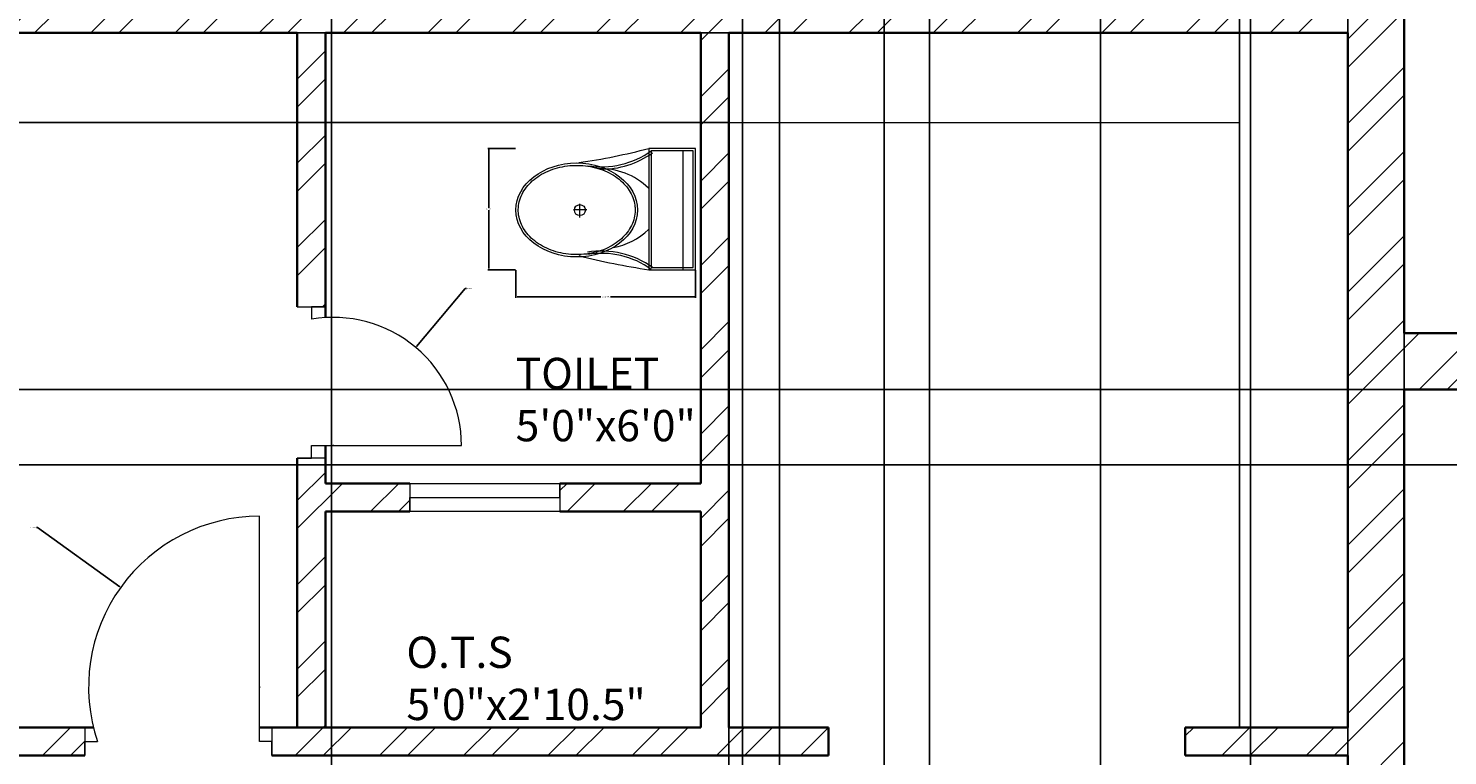
# Model space of a CAD drawing. Units: inches. Extents: x 1748 to 2382, y 1346 to 2284.
# Tile 11 of 26: x 1920 to 2147, y 1855 to 1971. Entities that reach past the tile are written whole.
import ezdxf

# ---------------------------------------------------------------- set-up
doc = ezdxf.new("R2010")
doc.units = ezdxf.units.IN
for name, color, linetype, lineweight in [('A-ANNO-DIMS', 2, 'Continuous', 18), ('A-AREA-IDEN', 7, 'Continuous', 18), ('A-DOOR', 21, 'Continuous', 18), ('A-FLOR-CASE', 32, 'Continuous', 18), ('A-FLOR-FIXT', 7, 'Continuous', 18), ('A-GLAZ', 191, 'Continuous', 18), ('A-WALL', 7, 'Continuous', 35), ('A-WALL-PATT', 9, 'Continuous', 13)]:
    doc.layers.add(name, color=color, linetype=linetype, lineweight=lineweight)
doc.styles.get("Standard").update_dxf_attribs({"font": 'arial.ttf'})
doc.dimstyles.get("Standard").update_dxf_attribs({"dimtxt": 0.18, "dimasz": 0.18, "dimexe": 0.18, "dimexo": 0.0625, "dimgap": 0.09, "dimtad": 0, "dimtih": 1, "dimtoh": 1, "dimdec": 4, "dimzin": 0, "dimdsep": 46, "dimtxsty": 'Standard', "dimcen": 0.09, "dimadec": 0, "dimazin": 0, "dimtfac": 1, "dimtdec": 4, "dimtofl": 0, "dimtmove": 0, "dimatfit": 3, "dimfxl": 1, "dimtolj": 1, "dimtzin": 0, "dimarcsym": 0})

# ---------------------------------------------------------------- blocks, each defined once
blk = doc.blocks.new('A$C31115884')
for p, q in [((283.1, 497.7), (223.4, 497.7)), ((257.5, 466.4), (257.5, 523.2)), ((0, 200), (0, 0)), ((520, 200), (0, 200)), ((10, 190), (10, 10)), ((510, 190), (10, 190)), ((510, 10), (510, 190)), ((520, 0), (520, 200)), ((510, 54.5), (0, 54.5)), ((10, 10), (510, 10)), ((0, 0), (520, 0))]:
    blk.add_line(p, q)
blk.add_circle((255.6, 496.4), 23.6)
for centre, radius, start, end in [((2777.7, -204.6), 2807, 165.4549, 171.71327), ((3237, 905), 2807, 188.28673, 194.5451), ((-294.5, 403.3), 364.7, 324.20913, 9.34987), ((-294.5, 403.3), 374.7, 324.20913, 9.34987), ((805.8, 403.3), 364.7, 170.65013, 215.79087), ((139.5, 406.2), 293.5, 315.84364, 2.65635), ((805.8, 403.3), 374.7, 179.20365, 215.79087), ((383.6, 406.2), 293.5, 190.27735, 224.15636)]:
    blk.add_arc(centre, radius, start, end)
blk.add_ellipse((256.2, 509.9), major_axis=(0, -260.7), ratio=0.772727)
blk.add_open_spline([(256.2, 259.2), (263.1, 259.2), (270, 259.7), (287.8, 262.3), (298.7, 265.1), (319.9, 273.1), (330.2, 278.4), (350.1, 291.1), (359.7, 298.7), (377.7, 315.9), (386.2, 325.5), (401.7, 346.6), (408.8, 358.1), (421.3, 382.5), (426.8, 395.5), (435.9, 422.4), (439.5, 436.4), (444.8, 465.1), (446.5, 479.7), (447.9, 509.2), (447.6, 524), (445, 553.3), (442.7, 567.8), (436.3, 596), (432.1, 609.7), (421.9, 636), (416, 648.6), (402.5, 672.1), (395, 683), (378.6, 703), (369.8, 712.1), (351.1, 728), (341.3, 734.8), (320.9, 746.2), (310.4, 750.7), (288.9, 757.3), (278, 759.4), (256, 761), (245, 760.6), (223.1, 757.2), (212.3, 754.3), (191.1, 746.1), (180.8, 740.7), (160.9, 727.8), (151.4, 720.1), (133.5, 702.7), (125.1, 693), (109.6, 671.7), (102.6, 660.2), (90.2, 635.7), (84.9, 622.7), (76, 595.6), (72.4, 581.6), (67.2, 552.9), (65.6, 538.2), (64.4, 508.8), (64.8, 494), (67.5, 464.7), (69.9, 450.2), (76.6, 422), (80.8, 408.3), (91.1, 382.2), (97.2, 369.7), (110.8, 346.3), (118.4, 335.4), (134.8, 315.6), (143.7, 306.7), (162.4, 290.9), (172.3, 284.2), (192.8, 273), (203.3, 268.6), (224.8, 262.2), (235.8, 260.2), (249.9, 259.3), (253, 259.2), (256.2, 259.2)], degree=3, knots=[0, 0, 0, 0, 0.110105, 0.110105, 0.285049, 0.285049, 0.459994, 0.459994, 0.634938, 0.634938, 0.809882, 0.809882, 0.984827, 0.984827, 1.159771, 1.159771, 1.334715, 1.334715, 1.50966, 1.50966, 1.684604, 1.684604, 1.859549, 1.859549, 2.034493, 2.034493, 2.209437, 2.209437, 2.384382, 2.384382, 2.559326, 2.559326, 2.73427, 2.73427, 2.909215, 2.909215, 3.084159, 3.084159, 3.259103, 3.259103, 3.434048, 3.434048, 3.608992, 3.608992, 3.783936, 3.783936, 3.958881, 3.958881, 4.133825, 4.133825, 4.30877, 4.30877, 4.483714, 4.483714, 4.658658, 4.658658, 4.833603, 4.833603, 5.008547, 5.008547, 5.183491, 5.183491, 5.358436, 5.358436, 5.53338, 5.53338, 5.708324, 5.708324, 5.883269, 5.883269, 6.058213, 6.058213, 6.233158, 6.233158, 6.283185, 6.283185, 6.283185, 6.283185])
blk = doc.blocks.new('*D14')
at = {"layer": 'A-ANNO-DIMS', "color": 0, "lineweight": -2, "transparency": 16777216}
for p, q in [((1997.92, 1932.42), (1997.92, 1928)), ((2026.64, 1932.42), (2026.64, 1928)), ((1998.1, 1928.18), (2011.5, 1928.18)), ((2026.46, 1928.18), (2013.06, 1928.18))]:
    blk.add_line(p, q, dxfattribs=at)
at = {"layer": 'A-ANNO-DIMS', "color": 0, "transparency": 16777216}
for points in [[(1998.1, 1928.21), (1998.1, 1928.15), (1997.92, 1928.18)], [(2026.46, 1928.21), (2026.46, 1928.15), (2026.64, 1928.18)]]:
    blk.add_solid(points, dxfattribs=at)
at = {"layer": 'Defpoints', "color": 0, "transparency": 16777216}
for p in [(1997.92, 1932.48), (2026.64, 1932.48), (1997.92, 1928.18)]:
    blk.add_point(p, dxfattribs=at)
at = {"layer": 'A-ANNO-DIMS', "color": 0, "transparency": 16777216, "insert": (2012.28, 1928.18), "char_height": 0.18, "attachment_point": 5}
blk.add_mtext('\\A1;WC 29 TYP.', dxfattribs=at)
blk = doc.blocks.new('*D15')
at = {"layer": 'A-ANNO-DIMS', "color": 0, "lineweight": -2, "transparency": 16777216}
for p, q in [((1997.86, 1951.87), (1993.43, 1951.87)), ((1993.61, 1951.69), (1993.61, 1942.36)), ((1993.61, 1932.66), (1993.61, 1941.99)), ((1997.86, 1932.48), (1993.43, 1932.48))]:
    blk.add_line(p, q, dxfattribs=at)
at = {"layer": 'A-ANNO-DIMS', "color": 0, "transparency": 16777216}
for points in [[(1993.58, 1951.69), (1993.64, 1951.69), (1993.61, 1951.87)], [(1993.58, 1932.66), (1993.64, 1932.66), (1993.61, 1932.48)]]:
    blk.add_solid(points, dxfattribs=at)
at = {"layer": 'Defpoints', "color": 0, "transparency": 16777216}
for p in [(1993.61, 1951.87), (1997.92, 1951.87), (1997.92, 1932.48)]:
    blk.add_point(p, dxfattribs=at)
at = {"layer": 'A-ANNO-DIMS', "color": 0, "transparency": 16777216, "insert": (1993.61, 1942.18), "char_height": 0.18, "attachment_point": 5}
blk.add_mtext('\\A1;19 TYP.', dxfattribs=at)
blk = doc.blocks.new('*D36')
at = {"layer": 'A-ANNO-DIMS', "color": 0, "lineweight": -2, "transparency": 16777216}
for p, q in [((2031.96, 1970.29), (2031.96, 1360.47)), ((2130.96, 1970.29), (2130.96, 1360.47)), ((2032.14, 1360.65), (2081.24, 1360.65)), ((2130.78, 1360.65), (2081.68, 1360.65))]:
    blk.add_line(p, q, dxfattribs=at)
at = {"layer": 'A-ANNO-DIMS', "color": 0, "transparency": 16777216}
for points in [[(2032.14, 1360.68), (2032.14, 1360.62), (2031.96, 1360.65)], [(2130.78, 1360.68), (2130.78, 1360.62), (2130.96, 1360.65)]]:
    blk.add_solid(points, dxfattribs=at)
at = {"layer": 'Defpoints', "color": 0, "transparency": 16777216}
for p in [(2031.96, 1970.35), (2130.96, 1970.35), (2130.96, 1360.65)]:
    blk.add_point(p, dxfattribs=at)
at = {"layer": 'A-ANNO-DIMS', "color": 0, "transparency": 16777216, "insert": (2081.46, 1360.65), "char_height": 0.18, "attachment_point": 5}
blk.add_mtext('\\A1;99', dxfattribs=at)
blk = doc.blocks.new('*D37')
at = {"layer": 'A-ANNO-DIMS', "color": 0, "lineweight": -2, "transparency": 16777216}
for p, q in [((2031.9, 1970.35), (1779.88, 1970.35)), ((1780.06, 1970.17), (1780.06, 1963.37)), ((1780.06, 1956.2), (1780.06, 1963.01)), ((2031.9, 1956.02), (1779.88, 1956.02))]:
    blk.add_line(p, q, dxfattribs=at)
at = {"layer": 'A-ANNO-DIMS', "color": 0, "transparency": 16777216}
for points in [[(1780.03, 1970.17), (1780.09, 1970.17), (1780.06, 1970.35)], [(1780.03, 1956.2), (1780.09, 1956.2), (1780.06, 1956.02)]]:
    blk.add_solid(points, dxfattribs=at)
at = {"layer": 'Defpoints', "color": 0, "transparency": 16777216}
for p in [(1780.06, 1970.35), (2031.96, 1970.35), (2031.96, 1956.02)]:
    blk.add_point(p, dxfattribs=at)
at = {"layer": 'A-ANNO-DIMS', "color": 0, "transparency": 16777216, "insert": (1780.06, 1963.19), "char_height": 0.18, "attachment_point": 5}
blk.add_mtext('\\A1;14.325', dxfattribs=at)
blk = doc.blocks.new('*D38')
at = {"layer": 'A-ANNO-DIMS', "color": 0, "lineweight": -2, "transparency": 16777216}
for p, q in [((2113.63, 1859.41), (2113.63, 2274.93)), ((2113.81, 2274.75), (2121.84, 2274.75)), ((2130.78, 2274.75), (2122.75, 2274.75)), ((2130.96, 1859.41), (2130.96, 2274.93))]:
    blk.add_line(p, q, dxfattribs=at)
at = {"layer": 'A-ANNO-DIMS', "color": 0, "transparency": 16777216}
for points in [[(2113.81, 2274.78), (2113.81, 2274.72), (2113.63, 2274.75)], [(2130.78, 2274.78), (2130.78, 2274.72), (2130.96, 2274.75)]]:
    blk.add_solid(points, dxfattribs=at)
at = {"layer": 'Defpoints', "color": 0, "transparency": 16777216}
for p in [(2130.96, 2274.75), (2113.63, 1859.35), (2130.96, 1859.35)]:
    blk.add_point(p, dxfattribs=at)
at = {"layer": 'A-ANNO-DIMS', "color": 0, "transparency": 16777216, "insert": (2122.29, 2274.75), "char_height": 0.18, "attachment_point": 5}
blk.add_mtext('\\A1;17.334', dxfattribs=at)
blk = doc.blocks.new('*D39')
at = {"layer": 'A-ANNO-DIMS', "color": 0, "lineweight": -2, "transparency": 16777216}
for p, q in [((2139.96, 1734.91), (2139.96, 2274.93)), ((2140.14, 2274.75), (2168.14, 2274.75)), ((2196.89, 2274.75), (2168.89, 2274.75)), ((2197.07, 1734.91), (2197.07, 2274.93))]:
    blk.add_line(p, q, dxfattribs=at)
at = {"layer": 'A-ANNO-DIMS', "color": 0, "transparency": 16777216}
for points in [[(2140.14, 2274.78), (2140.14, 2274.72), (2139.96, 2274.75)], [(2196.89, 2274.78), (2196.89, 2274.72), (2197.07, 2274.75)]]:
    blk.add_solid(points, dxfattribs=at)
at = {"layer": 'Defpoints', "color": 0, "transparency": 16777216}
for p in [(2197.07, 2274.75), (2139.96, 1734.85), (2197.07, 1734.85)]:
    blk.add_point(p, dxfattribs=at)
at = {"layer": 'A-ANNO-DIMS', "color": 0, "transparency": 16777216, "insert": (2168.52, 2274.75), "char_height": 0.18, "attachment_point": 5}
blk.add_mtext('\\A1;57.11', dxfattribs=at)
blk = doc.blocks.new('*D51')
at = {"layer": 'A-ANNO-DIMS', "color": 0, "lineweight": -2, "transparency": 16777216}
for p, q in [((1968.44, 2223.79), (1968.44, 1360.47)), ((2040.07, 2223.79), (2040.07, 1360.47)), ((1968.62, 1360.65), (2003.86, 1360.65)), ((2039.89, 1360.65), (2004.65, 1360.65))]:
    blk.add_line(p, q, dxfattribs=at)
at = {"layer": 'A-ANNO-DIMS', "color": 0, "transparency": 16777216}
for points in [[(1968.62, 1360.68), (1968.62, 1360.62), (1968.44, 1360.65)], [(2039.89, 1360.68), (2039.89, 1360.62), (2040.07, 1360.65)]]:
    blk.add_solid(points, dxfattribs=at)
at = {"layer": 'Defpoints', "color": 0, "transparency": 16777216}
for p in [(1968.44, 2223.85), (2040.07, 2223.85), (2040.07, 1360.65)]:
    blk.add_point(p, dxfattribs=at)
at = {"layer": 'A-ANNO-DIMS', "color": 0, "transparency": 16777216, "insert": (2004.26, 1360.65), "char_height": 0.18, "attachment_point": 5}
blk.add_mtext('\\A1;71.62', dxfattribs=at)
blk = doc.blocks.new('*D52')
at = {"layer": 'A-ANNO-DIMS', "color": 0, "lineweight": -2, "transparency": 16777216}
for p, q in [((2064.07, 2223.79), (2064.07, 1360.47)), ((2091.4, 2223.79), (2091.4, 1360.47)), ((2064.25, 1360.65), (2077.34, 1360.65)), ((2091.22, 1360.65), (2078.13, 1360.65))]:
    blk.add_line(p, q, dxfattribs=at)
at = {"layer": 'A-ANNO-DIMS', "color": 0, "transparency": 16777216}
for points in [[(2064.25, 1360.68), (2064.25, 1360.62), (2064.07, 1360.65)], [(2091.22, 1360.68), (2091.22, 1360.62), (2091.4, 1360.65)]]:
    blk.add_solid(points, dxfattribs=at)
at = {"layer": 'Defpoints', "color": 0, "transparency": 16777216}
for p in [(2064.07, 2223.85), (2091.4, 2223.85), (2091.4, 1360.65)]:
    blk.add_point(p, dxfattribs=at)
at = {"layer": 'A-ANNO-DIMS', "color": 0, "transparency": 16777216, "insert": (2077.73, 1360.65), "char_height": 0.18, "attachment_point": 5}
blk.add_mtext('\\A1;27.33', dxfattribs=at)
blk = doc.blocks.new('*D53')
at = {"layer": 'A-ANNO-DIMS', "color": 0, "lineweight": -2, "transparency": 16777216}
for p, q in [((2115.4, 2223.79), (2115.4, 1360.47)), ((2167.02, 2223.79), (2167.02, 1360.47)), ((2115.58, 1360.65), (2140.81, 1360.65)), ((2166.84, 1360.65), (2141.6, 1360.65))]:
    blk.add_line(p, q, dxfattribs=at)
at = {"layer": 'A-ANNO-DIMS', "color": 0, "transparency": 16777216}
for points in [[(2115.58, 1360.68), (2115.58, 1360.62), (2115.4, 1360.65)], [(2166.84, 1360.68), (2166.84, 1360.62), (2167.02, 1360.65)]]:
    blk.add_solid(points, dxfattribs=at)
at = {"layer": 'Defpoints', "color": 0, "transparency": 16777216}
for p in [(2115.4, 2223.85), (2167.02, 2223.85), (2167.02, 1360.65)]:
    blk.add_point(p, dxfattribs=at)
at = {"layer": 'A-ANNO-DIMS', "color": 0, "transparency": 16777216, "insert": (2141.21, 1360.65), "char_height": 0.18, "attachment_point": 5}
blk.add_mtext('\\A1;51.62', dxfattribs=at)
blk = doc.blocks.new('*D56')
at = {"layer": 'A-ANNO-DIMS', "color": 0, "lineweight": -2, "transparency": 16777216}
for p, q in [((2288.4, 1913.35), (1779.88, 1913.35)), ((1780.06, 1913.17), (1780.06, 1907.52)), ((1780.06, 1901.51), (1780.06, 1907.16)), ((2288.4, 1901.33), (1779.88, 1901.33))]:
    blk.add_line(p, q, dxfattribs=at)
at = {"layer": 'A-ANNO-DIMS', "color": 0, "transparency": 16777216}
for points in [[(1780.03, 1913.17), (1780.09, 1913.17), (1780.06, 1913.35)], [(1780.03, 1901.51), (1780.09, 1901.51), (1780.06, 1901.33)]]:
    blk.add_solid(points, dxfattribs=at)
at = {"layer": 'Defpoints', "color": 0, "transparency": 16777216}
for p in [(1780.06, 1913.35), (2288.46, 1913.35), (2288.46, 1901.33)]:
    blk.add_point(p, dxfattribs=at)
at = {"layer": 'A-ANNO-DIMS', "color": 0, "transparency": 16777216, "insert": (1780.06, 1907.34), "char_height": 0.18, "attachment_point": 5}
blk.add_mtext('\\A1;12.023', dxfattribs=at)
blk = doc.blocks.new('*D78')
at = {"layer": 'A-ANNO-DIMS', "color": 0, "lineweight": -2, "transparency": 16777216}
for p, q in [((2034.13, 2132.54), (2034.13, 1360.47)), ((2056.8, 2127.06), (2056.8, 1360.47)), ((2034.31, 1360.65), (2045, 1360.65)), ((2056.62, 1360.65), (2045.93, 1360.65))]:
    blk.add_line(p, q, dxfattribs=at)
at = {"layer": 'A-ANNO-DIMS', "color": 0, "transparency": 16777216}
for points in [[(2034.31, 1360.68), (2034.31, 1360.62), (2034.13, 1360.65)], [(2056.62, 1360.68), (2056.62, 1360.62), (2056.8, 1360.65)]]:
    blk.add_solid(points, dxfattribs=at)
at = {"layer": 'Defpoints', "color": 0, "transparency": 16777216}
for p in [(2034.13, 2132.6), (2056.8, 2127.13), (2056.8, 1360.65)]:
    blk.add_point(p, dxfattribs=at)
at = {"layer": 'A-ANNO-DIMS', "color": 0, "transparency": 16777216, "insert": (2045.47, 1360.65), "char_height": 0.18, "attachment_point": 5}
blk.add_mtext('\\A1;22.663', dxfattribs=at)
blk = doc.blocks.new('*D84')
at = {"layer": 'A-ANNO-DIMS', "color": 0, "lineweight": -2, "transparency": 16777216}
for p, q in [((1921.24, 1891.31), (1921.42, 1891.31)), ((1921.42, 1891.31), (1934.58, 1881.84)), ((1956.81, 1865.78), (1956.99, 1865.78)), ((1956.9, 1865.69), (1956.9, 1865.87))]:
    blk.add_line(p, q, dxfattribs=at)
at = {"layer": 'A-ANNO-DIMS', "color": 0, "transparency": 16777216}
blk.add_solid([(1934.6, 1881.87), (1934.56, 1881.82), (1934.72, 1881.74)], dxfattribs=at)
at = {"layer": 'Defpoints', "color": 0, "transparency": 16777216}
for p in [(1934.72, 1881.74), (1956.9, 1865.78)]:
    blk.add_point(p, dxfattribs=at)
at = {"layer": 'A-ANNO-DIMS', "color": 0, "transparency": 16777216, "insert": (1920.69, 1891.31), "char_height": 0.18, "attachment_point": 5}
blk.add_mtext('\\A1;R27.315', dxfattribs=at)
blk = doc.blocks.new('*D89')
at = {"layer": 'A-ANNO-DIMS', "color": 0, "lineweight": -2, "transparency": 16777216}
for p, q in [((1989.82, 1929.47), (1982.03, 1920.2)), ((1990, 1929.47), (1989.82, 1929.47)), ((1968.63, 1904.38), (1968.81, 1904.38)), ((1968.72, 1904.29), (1968.72, 1904.47))]:
    blk.add_line(p, q, dxfattribs=at)
at = {"layer": 'A-ANNO-DIMS', "color": 0, "transparency": 16777216}
blk.add_solid([(1982, 1920.22), (1982.05, 1920.18), (1981.91, 1920.07)], dxfattribs=at)
at = {"layer": 'Defpoints', "color": 0, "transparency": 16777216}
for p in [(1981.91, 1920.07), (1968.72, 1904.38)]:
    blk.add_point(p, dxfattribs=at)
at = {"layer": 'A-ANNO-DIMS', "color": 0, "transparency": 16777216, "insert": (1990.48, 1929.47), "char_height": 0.18, "attachment_point": 5}
blk.add_mtext('\\A1;R20.49', dxfattribs=at)

msp = doc.modelspace()

# ---------------------------------------------------------------- hatches: boundary and pattern name
at = {"layer": 'A-WALL-PATT'}
h = msp.add_hatch(dxfattribs=at)
h.set_pattern_fill('ANSI32', color=256)
h.paths.add_polyline_path([(1908.4445, 2232.8497), (1821.9607, 2232.8497), (1821.9607, 2223.8497), (1865.4607, 2223.8497), (1865.4607, 2209.9185), (1869.9607, 2209.9185), (1869.9607, 2223.8497), (1908.4445, 2223.8497), (1908.4445, 2228.3497)])
h.paths.add_polyline_path([(2040.0683, 2232.8497), (1968.4445, 2232.8497), (1968.4445, 2223.8497), (2025.9607, 2223.8497), (2025.9607, 2130.3497), (2032.1341, 2130.3497), (2032.1341, 2132.5997), (2032.1341, 2134.8497), (2030.4607, 2134.8497), (2030.4607, 2223.8497), (2040.0683, 2223.8497)])
h.paths.add_polyline_path([(2091.3969, 2232.8497), (2064.0683, 2232.8497), (2064.0683, 2223.8497), (2078.4607, 2223.8497), (2078.4607, 2134.8497), (2051.1563, 2134.8497), (2051.1563, 2130.3497), (2078.4607, 2130.3497), (2078.4607, 2128.6813), (2082.9607, 2128.6813), (2082.9607, 2130.3497), (2086.1879, 2130.3497), (2086.1879, 2132.5997), (2086.1879, 2134.8497), (2082.9607, 2134.8497), (2082.9607, 2223.8497), (2091.3969, 2223.8497), (2091.3969, 2228.3497)])
h.paths.add_polyline_path([(2167.0164, 2232.8497), (2115.3969, 2232.8497), (2115.3969, 2223.8497), (2130.9607, 2223.8497), (2130.9607, 2134.8497), (2106.9607, 2134.8497), (2106.9607, 2130.3497), (2135.4607, 2130.3497), (2135.4607, 2223.8497), (2167.0164, 2223.8497), (2167.0164, 2228.3497)])
h.paths.add_polyline_path([(1869.9607, 2149.9185), (1865.4607, 2149.9185), (1865.4607, 2127.8942), (1869.9607, 2127.8942)])
h.paths.add_polyline_path([(2082.9607, 2104.4871), (2080.7107, 2104.4871), (2078.4607, 2104.4871), (2078.4607, 2103.8497), (1869.9607, 2103.8497), (1869.9607, 2108.6062), (1867.7107, 2108.6062), (1865.4607, 2108.6062), (1865.4607, 2103.8497), (1821.9607, 2103.8497), (1821.9607, 2099.3497), (1865.4607, 2099.3497), (1865.4607, 2094.7509), (1869.9607, 2094.7509), (1869.9607, 2099.3497), (2025.9607, 2099.3497), (2025.9607, 2096.4326), (2030.4607, 2096.4326), (2030.4607, 2099.3497), (2082.9607, 2099.3497)])
h.paths.add_polyline_path([(1928.9457, 1401.1212), (2176.8693, 1401.1212), (2176.8693, 1438.214), (1928.9457, 1438.214)], flags=9)
h.paths.add_polyline_path([(2122.2668, 2048.1927), (2177.9387, 2048.1927), (2177.9387, 2066.85), (2122.2668, 2066.85)], flags=9)
h.paths.add_polyline_path([(2272.688, 2153.8197), (2272.688, 2216.746), (2262.3845, 2216.746), (2262.3845, 2153.8197)], flags=9)
h.paths.add_polyline_path([(2157.2928, 2166.5593), (2196.3822, 2166.5593), (2196.3822, 2185.2167), (2157.2928, 2185.2167)], flags=9)
h.paths.add_polyline_path([(2089.3407, 2162.0698), (2124.3987, 2162.0698), (2124.3987, 2180.7272), (2089.3407, 2180.7272)], flags=9)
h.paths.add_polyline_path([(2037.4521, 2160.0913), (2072.5101, 2160.0913), (2072.5101, 2178.7486), (2037.4521, 2178.7486)], flags=9)
h.paths.add_polyline_path([(1884.7894, 2104.1554), (1923.6297, 2104.1554), (1923.6297, 2122.8127), (1884.7894, 2122.8127)], flags=9)
h.paths.add_polyline_path([(1851.2832, 2142.9749), (1851.2832, 2199.3051), (1840.9796, 2199.3051), (1840.9796, 2142.9749)], flags=9)
h.paths.add_polyline_path([(1844.8763, 2017.2834), (1844.8763, 2073.6136), (1834.5728, 2073.6136), (1834.5728, 2017.2834)], flags=9)
h.paths.add_polyline_path([(1897.1577, 2073.1279), (1935.9981, 2073.1279), (1935.9981, 2091.7853), (1897.1577, 2091.7853)], flags=9)
h.paths.add_polyline_path([(1952.3395, 1802.4231), (2008.0114, 1802.4231), (2008.0114, 1821.0805), (1952.3395, 1821.0805)], flags=9)
h.paths.add_polyline_path([(1978.8184, 1857.6841), (2017.7338, 1857.6841), (2017.7338, 1876.3415), (1978.8184, 1876.3415)], flags=9)
h.paths.add_polyline_path([(1979.6513, 1925.9516), (2008.8089, 1925.9516), (2008.8089, 1944.6089), (1979.6513, 1944.6089)], flags=9)
h.paths.add_polyline_path([(1838.5553, 1860.3527), (1877.3957, 1860.3527), (1877.3957, 1879.01), (1838.5553, 1879.01)], flags=9)
h.paths.add_polyline_path([(1883.9018, 1787.3013), (1883.9018, 1843.6315), (1873.5983, 1843.6315), (1873.5983, 1787.3013)], flags=9)
h.paths.add_polyline_path([(1873.7079, 1509.1938), (1873.7079, 1583.7709), (1863.4044, 1583.7709), (1863.4044, 1509.1938)], flags=9)
h.paths.add_polyline_path([(1916.2259, 1603.3681), (1955.0663, 1603.3681), (1955.0663, 1622.0254), (1916.2259, 1622.0254)], flags=9)
h.paths.add_polyline_path([(1876.3013, 1636.757), (1876.3013, 1693.0871), (1865.9978, 1693.0871), (1865.9978, 1636.757)], flags=9)
h.paths.add_polyline_path([(1921.3138, 1521.8316), (1964.0662, 1521.8316), (1964.0662, 1540.489), (1921.3138, 1540.489)], flags=9)
h.paths.add_polyline_path([(2017.5657, 1497.5078), (2046.7983, 1497.5078), (2046.7983, 1516.1651), (2017.5657, 1516.1651)], flags=9)
h.paths.add_polyline_path([(2066.8661, 1499.3902), (2096.0988, 1499.3902), (2096.0988, 1518.0475), (2066.8661, 1518.0475)], flags=9)
h.paths.add_polyline_path([(2155.4835, 1571.6596), (2198.2358, 1571.6596), (2198.2358, 1590.3169), (2155.4835, 1590.3169)], flags=9)
h.paths.add_polyline_path([(2094.9136, 1664.6812), (2150.5855, 1664.6812), (2150.5855, 1683.3386), (2094.9136, 1683.3386)], flags=9)
h.paths.add_polyline_path([(2257.6902, 1863.1628), (2269.8935, 1863.1628), (2269.8935, 1873.4664), (2257.6902, 1873.4664)], flags=9)
h.paths.add_polyline_path([(2164.0748, 1880.3089), (2189.8694, 1880.3089), (2189.8694, 1890.6124), (2164.0748, 1890.6124)], flags=9)
h.paths.add_polyline_path([(2239.4394, 1931.0585), (2268.8187, 1931.0585), (2268.8187, 1949.7159), (2239.4394, 1949.7159)], flags=9)
h = msp.add_hatch(dxfattribs=at)
h.set_pattern_fill('ANSI32', color=256)
h.paths.add_polyline_path([(2297.4607, 2232.8497), (2203.0164, 2232.8497), (2203.0164, 2223.8497), (2244.9607, 2223.8497), (2244.9607, 2127.8554), (2249.4607, 2127.8554), (2249.4607, 2223.8497), (2297.4607, 2223.8497)])
h.paths.add_polyline_path([(2297.4607, 2103.8497), (2249.4607, 2103.8497), (2249.4607, 2106.7497), (2247.2107, 2106.7497), (2244.9607, 2106.7497), (2244.9607, 2103.8497), (2130.9607, 2103.8497), (2130.9607, 2099.3497), (2288.4607, 2099.3497), (2288.4607, 2077.2008), (2297.4607, 2077.2008)])
h.paths.add_polyline_path([(1928.9457, 1401.1212), (2176.8693, 1401.1212), (2176.8693, 1438.214), (1928.9457, 1438.214)], flags=9)
h.paths.add_polyline_path([(2122.2668, 2048.1927), (2177.9387, 2048.1927), (2177.9387, 2066.85), (2122.2668, 2066.85)], flags=9)
h.paths.add_polyline_path([(2272.688, 2153.8197), (2272.688, 2216.746), (2262.3845, 2216.746), (2262.3845, 2153.8197)], flags=25)
h.paths.add_polyline_path([(2157.2928, 2166.5593), (2196.3822, 2166.5593), (2196.3822, 2185.2167), (2157.2928, 2185.2167)], flags=9)
h.paths.add_polyline_path([(2089.3407, 2162.0698), (2124.3987, 2162.0698), (2124.3987, 2180.7272), (2089.3407, 2180.7272)], flags=9)
h.paths.add_polyline_path([(2037.4521, 2160.0913), (2072.5101, 2160.0913), (2072.5101, 2178.7486), (2037.4521, 2178.7486)], flags=9)
h.paths.add_polyline_path([(1884.7894, 2104.1554), (1923.6297, 2104.1554), (1923.6297, 2122.8127), (1884.7894, 2122.8127)], flags=9)
h.paths.add_polyline_path([(1851.2832, 2142.9749), (1851.2832, 2199.3051), (1840.9796, 2199.3051), (1840.9796, 2142.9749)], flags=9)
h.paths.add_polyline_path([(1844.8763, 2017.2834), (1844.8763, 2073.6136), (1834.5728, 2073.6136), (1834.5728, 2017.2834)], flags=9)
h.paths.add_polyline_path([(1897.1577, 2073.1279), (1935.9981, 2073.1279), (1935.9981, 2091.7853), (1897.1577, 2091.7853)], flags=9)
h.paths.add_polyline_path([(1952.3395, 1802.4231), (2008.0114, 1802.4231), (2008.0114, 1821.0805), (1952.3395, 1821.0805)], flags=9)
h.paths.add_polyline_path([(1978.8184, 1857.6841), (2017.7338, 1857.6841), (2017.7338, 1876.3415), (1978.8184, 1876.3415)], flags=9)
h.paths.add_polyline_path([(1979.6513, 1925.9516), (2008.8089, 1925.9516), (2008.8089, 1944.6089), (1979.6513, 1944.6089)], flags=9)
h.paths.add_polyline_path([(1838.5553, 1860.3527), (1877.3957, 1860.3527), (1877.3957, 1879.01), (1838.5553, 1879.01)], flags=9)
h.paths.add_polyline_path([(1883.9018, 1787.3013), (1883.9018, 1843.6315), (1873.5983, 1843.6315), (1873.5983, 1787.3013)], flags=9)
h.paths.add_polyline_path([(1873.7079, 1509.1938), (1873.7079, 1583.7709), (1863.4044, 1583.7709), (1863.4044, 1509.1938)], flags=9)
h.paths.add_polyline_path([(1916.2259, 1603.3681), (1955.0663, 1603.3681), (1955.0663, 1622.0254), (1916.2259, 1622.0254)], flags=9)
h.paths.add_polyline_path([(1876.3013, 1636.757), (1876.3013, 1693.0871), (1865.9978, 1693.0871), (1865.9978, 1636.757)], flags=9)
h.paths.add_polyline_path([(1921.3138, 1521.8316), (1964.0662, 1521.8316), (1964.0662, 1540.489), (1921.3138, 1540.489)], flags=9)
h.paths.add_polyline_path([(2017.5657, 1497.5078), (2046.7983, 1497.5078), (2046.7983, 1516.1651), (2017.5657, 1516.1651)], flags=9)
h.paths.add_polyline_path([(2066.8661, 1499.3902), (2096.0988, 1499.3902), (2096.0988, 1518.0475), (2066.8661, 1518.0475)], flags=9)
h.paths.add_polyline_path([(2155.4835, 1571.6596), (2198.2358, 1571.6596), (2198.2358, 1590.3169), (2155.4835, 1590.3169)], flags=9)
h.paths.add_polyline_path([(2094.9136, 1664.6812), (2150.5855, 1664.6812), (2150.5855, 1683.3386), (2094.9136, 1683.3386)], flags=9)
h.paths.add_polyline_path([(2257.6902, 1863.1628), (2269.8935, 1863.1628), (2269.8935, 1873.4664), (2257.6902, 1873.4664)], flags=9)
h.paths.add_polyline_path([(2164.0748, 1880.3089), (2189.8694, 1880.3089), (2189.8694, 1890.6124), (2164.0748, 1890.6124)], flags=9)
h.paths.add_polyline_path([(2239.4394, 1931.0585), (2268.8187, 1931.0585), (2268.8187, 1949.7159), (2239.4394, 1949.7159)], flags=9)
h = msp.add_hatch(dxfattribs=at)
h.set_pattern_fill('ANSI32', color=256)
h.paths.add_polyline_path([(1919.6777, 1476.8497), (1900.6426, 1476.8497), (1900.6426, 1522.0826), (1898.3926, 1522.0826), (1896.1426, 1522.0826), (1896.1426, 1476.8497), (1857.1426, 1476.8497), (1857.1426, 1467.8497), (1896.1426, 1467.8497), (1919.6777, 1467.8497), (1919.6777, 1472.3497)])
h.paths.add_polyline_path([(2018.7873, 1472.3497), (2018.7873, 1476.8497), (2010.9607, 1476.8497), (2010.9607, 1560.8497), (2034.9607, 1560.8497), (2034.9607, 1565.3497), (2006.4607, 1565.3497), (2006.4607, 1476.8497), (1955.6777, 1476.8497), (1955.6777, 1467.8497), (2018.7873, 1467.8497)])
h.paths.add_polyline_path([(2152.3354, 1472.3497), (2152.3354, 1476.8497), (2115.9607, 1476.8497), (2115.9607, 1565.3497), (2109.2204, 1565.3497), (2109.2204, 1563.0997), (2109.2204, 1560.8497), (2111.4607, 1560.8497), (2111.4607, 1476.8497), (2095.3617, 1476.8497), (2095.3617, 1467.8497), (2152.3354, 1467.8497)])
h.paths.add_polyline_path([(2071.3617, 1476.8497), (2063.4607, 1476.8497), (2063.4607, 1560.8497), (2090.1865, 1560.8497), (2090.1865, 1565.3497), (2063.4607, 1565.3497), (2063.4607, 1572.5485), (2061.2107, 1572.5485), (2058.9607, 1572.5485), (2058.9607, 1565.3497), (2055.6281, 1565.3497), (2055.6281, 1560.8497), (2058.9607, 1560.8497), (2058.9607, 1476.8497), (2042.7873, 1476.8497), (2042.7873, 1467.8497), (2071.3617, 1467.8497), (2071.3617, 1472.3497)])
h.paths.add_polyline_path([(2297.4607, 1506.5652), (2288.4607, 1506.5652), (2288.4607, 1476.8497), (2212.3354, 1476.8497), (2212.3354, 1467.8497), (2297.4607, 1467.8497)])
h.paths.add_polyline_path([(2297.4607, 1645.3038), (2288.4607, 1645.3038), (2288.4607, 1605.8497), (2058.9607, 1605.8497), (2058.9607, 1600.1857), (2061.2107, 1600.1857), (2063.4607, 1600.1857), (2063.4607, 1601.3497), (2288.4607, 1601.3497), (2288.4607, 1566.5652), (2297.4607, 1566.5652)])
h.paths.add_polyline_path([(2010.9607, 1609.0561), (2008.7107, 1609.0561), (2006.4607, 1609.0561), (2006.4607, 1605.8497), (1900.6426, 1605.8497), (1900.6426, 1609.7171), (1898.3926, 1609.7171), (1896.1426, 1609.7171), (1896.1426, 1605.8497), (1857.1426, 1605.8497), (1857.1426, 1601.3497), (1896.1426, 1601.3497), (1896.1426, 1542.5447), (1900.6426, 1542.5447), (1900.6426, 1601.3497), (2010.9607, 1601.3497)])
h.paths.add_polyline_path([(1928.9457, 1401.1212), (2176.8693, 1401.1212), (2176.8693, 1438.214), (1928.9457, 1438.214)], flags=9)
h.paths.add_polyline_path([(2122.2668, 2048.1927), (2177.9387, 2048.1927), (2177.9387, 2066.85), (2122.2668, 2066.85)], flags=9)
h.paths.add_polyline_path([(2272.688, 2153.8197), (2272.688, 2216.746), (2262.3845, 2216.746), (2262.3845, 2153.8197)], flags=9)
h.paths.add_polyline_path([(2157.2928, 2166.5593), (2196.3822, 2166.5593), (2196.3822, 2185.2167), (2157.2928, 2185.2167)], flags=9)
h.paths.add_polyline_path([(2089.3407, 2162.0698), (2124.3987, 2162.0698), (2124.3987, 2180.7272), (2089.3407, 2180.7272)], flags=9)
h.paths.add_polyline_path([(2037.4521, 2160.0913), (2072.5101, 2160.0913), (2072.5101, 2178.7486), (2037.4521, 2178.7486)], flags=9)
h.paths.add_polyline_path([(1884.7894, 2104.1554), (1923.6297, 2104.1554), (1923.6297, 2122.8127), (1884.7894, 2122.8127)], flags=9)
h.paths.add_polyline_path([(1851.2832, 2142.9749), (1851.2832, 2199.3051), (1840.9796, 2199.3051), (1840.9796, 2142.9749)], flags=9)
h.paths.add_polyline_path([(1844.8763, 2017.2834), (1844.8763, 2073.6136), (1834.5728, 2073.6136), (1834.5728, 2017.2834)], flags=9)
h.paths.add_polyline_path([(1897.1577, 2073.1279), (1935.9981, 2073.1279), (1935.9981, 2091.7853), (1897.1577, 2091.7853)], flags=9)
h.paths.add_polyline_path([(1952.3395, 1802.4231), (2008.0114, 1802.4231), (2008.0114, 1821.0805), (1952.3395, 1821.0805)], flags=9)
h.paths.add_polyline_path([(1978.8184, 1857.6841), (2017.7338, 1857.6841), (2017.7338, 1876.3415), (1978.8184, 1876.3415)], flags=9)
h.paths.add_polyline_path([(1979.6513, 1925.9516), (2008.8089, 1925.9516), (2008.8089, 1944.6089), (1979.6513, 1944.6089)], flags=9)
h.paths.add_polyline_path([(1838.5553, 1860.3527), (1877.3957, 1860.3527), (1877.3957, 1879.01), (1838.5553, 1879.01)], flags=9)
h.paths.add_polyline_path([(1883.9018, 1787.3013), (1883.9018, 1843.6315), (1873.5983, 1843.6315), (1873.5983, 1787.3013)], flags=9)
h.paths.add_polyline_path([(1873.7079, 1509.1938), (1873.7079, 1583.7709), (1863.4044, 1583.7709), (1863.4044, 1509.1938)], flags=9)
h.paths.add_polyline_path([(1916.2259, 1603.3681), (1955.0663, 1603.3681), (1955.0663, 1622.0254), (1916.2259, 1622.0254)], flags=9)
h.paths.add_polyline_path([(1876.3013, 1636.757), (1876.3013, 1693.0871), (1865.9978, 1693.0871), (1865.9978, 1636.757)], flags=9)
h.paths.add_polyline_path([(1921.3138, 1521.8316), (1964.0662, 1521.8316), (1964.0662, 1540.489), (1921.3138, 1540.489)], flags=9)
h.paths.add_polyline_path([(2017.5657, 1497.5078), (2046.7983, 1497.5078), (2046.7983, 1516.1651), (2017.5657, 1516.1651)], flags=9)
h.paths.add_polyline_path([(2066.8661, 1499.3902), (2096.0988, 1499.3902), (2096.0988, 1518.0475), (2066.8661, 1518.0475)], flags=9)
h.paths.add_polyline_path([(2155.4835, 1571.6596), (2198.2358, 1571.6596), (2198.2358, 1590.3169), (2155.4835, 1590.3169)], flags=25)
h.paths.add_polyline_path([(2094.9136, 1664.6812), (2150.5855, 1664.6812), (2150.5855, 1683.3386), (2094.9136, 1683.3386)], flags=9)
h.paths.add_polyline_path([(2257.6902, 1863.1628), (2269.8935, 1863.1628), (2269.8935, 1873.4664), (2257.6902, 1873.4664)], flags=9)
h.paths.add_polyline_path([(2164.0748, 1880.3089), (2189.8694, 1880.3089), (2189.8694, 1890.6124), (2164.0748, 1890.6124)], flags=9)
h.paths.add_polyline_path([(2239.4394, 1931.0585), (2268.8187, 1931.0585), (2268.8187, 1949.7159), (2239.4394, 1949.7159)], flags=9)
h = msp.add_hatch(dxfattribs=at)
h.set_pattern_fill('ANSI32', color=256)
h.paths.add_polyline_path([(1900.6426, 1652.723), (1896.1426, 1652.723), (1896.1426, 1629.9029), (1900.6426, 1629.9029)])
h.paths.add_polyline_path([(2206.0699, 1859.3497), (2197.0699, 1859.3497), (2197.0699, 1734.8497), (2206.0699, 1734.8497)], flags=17)
h.paths.add_polyline_path([(2297.4607, 1865.3269), (2288.4607, 1865.3269), (2288.4607, 1734.8497), (2206.0699, 1734.8497), (2180.4551, 1734.8497), (2180.4551, 1725.8497), (2197.0699, 1725.8497), (2206.0699, 1725.8497), (2288.4607, 1725.8497), (2288.4607, 1705.3038), (2297.4607, 1705.3038)])
h.paths.add_polyline_path([(2139.9607, 1815.8001), (2135.4607, 1815.8001), (2130.9607, 1815.8001), (2130.9607, 1734.8497), (1900.6426, 1734.8497), (1900.6426, 1738.9477), (1898.3926, 1738.9477), (1896.1426, 1738.9477), (1896.1426, 1734.8497), (1857.1426, 1734.8497), (1857.1426, 1725.8497), (1896.1426, 1725.8497), (1896.1426, 1712.723), (1900.6426, 1712.723), (1900.6426, 1725.8497), (2006.4607, 1725.8497), (2006.4607, 1637.448), (2010.9607, 1637.448), (2010.9607, 1725.8497), (2139.9607, 1725.8497), (2147.389, 1725.8497), (2147.389, 1730.3497), (2147.389, 1734.8497), (2139.9607, 1734.8497)])
h.paths.add_polyline_path([(2149.8497, 1917.8497), (2149.8497, 1922.3497), (2139.9607, 1922.3497), (2139.9607, 1979.3497), (2030.4607, 1979.3497), (2030.4607, 2069.8971), (2028.2107, 2069.8971), (2025.9607, 2069.8971), (2025.9607, 1979.3497), (1869.9607, 1979.3497), (1869.9607, 1998.93), (1865.4607, 1998.93), (1865.4607, 1979.3497), (1821.9607, 1979.3497), (1821.9607, 1952.7922), (1826.9306, 1952.7922), (1830.9607, 1952.7922), (1830.9607, 1970.3497), (1962.9607, 1970.3497), (1962.9607, 1926.5713), (1967.4607, 1926.5713), (1967.4607, 1970.3497), (2027.4607, 1970.3497), (2027.4607, 1898.3497), (2004.9604, 1898.3497), (2004.9604, 1893.8497), (2027.4607, 1893.8497), (2027.4607, 1859.3497), (1958.8973, 1859.3497), (1958.8973, 1854.8497), (2047.917, 1854.8497), (2047.917, 1859.3497), (2031.9607, 1859.3497), (2031.9607, 1970.3497), (2130.9607, 1970.3497), (2130.9607, 1859.3497), (2104.9565, 1859.3497), (2104.9565, 1854.8497), (2130.9607, 1854.8497), (2130.9607, 1849.0684), (2139.9607, 1849.0684), (2139.9607, 1913.3497), (2149.8497, 1913.3497)])
h.paths.add_polyline_path([(1928.9996, 1859.3497), (1830.9607, 1859.3497), (1830.9607, 1892.7922), (1821.9607, 1892.7922), (1821.9607, 1854.8497), (1896.1426, 1854.8497), (1896.1426, 1836.6443), (1898.378, 1836.6443), (1900.6426, 1836.6443), (1900.6426, 1854.8497), (1928.9996, 1854.8497), (1928.9996, 1857.0997)])
h.paths.add_polyline_path([(1980.9604, 1896.0997), (1980.9604, 1898.3497), (1967.4607, 1898.3497), (1967.4607, 1902.3846), (1962.9607, 1902.3846), (1962.9607, 1859.3497), (1967.4607, 1859.3497), (1967.4607, 1893.8497), (1980.9604, 1893.8497)], flags=17)
h.paths.add_polyline_path([(1900.6426, 1776.6443), (1896.1426, 1776.6443), (1896.1426, 1758.0891), (1900.6426, 1758.0891)], flags=17)
h.paths.add_polyline_path([(2297.4607, 2017.2008), (2288.4607, 2017.2008), (2288.4607, 1979.3497), (2213.4607, 1979.3497), (2213.4607, 1922.3497), (2183.3516, 1922.3497), (2183.3516, 1913.3497), (2213.4607, 1913.3497), (2236.234, 1913.3497), (2236.234, 1922.3497), (2222.4607, 1922.3497), (2222.4607, 1931.3497), (2222.4607, 1970.3497), (2288.4607, 1970.3497), (2288.4607, 1922.3497), (2272.1921, 1922.3497), (2272.1921, 1913.3497), (2288.4607, 1913.3497), (2288.4607, 1901.3269), (2297.4607, 1901.3269)])

# ---------------------------------------------------------------- linework, layer by layer
at = {"layer": 'A-DOOR'}
for p, q in [((1962.9607, 1926.5713), (1967.4607, 1926.5713)), ((1967.4607, 1926.5713), (1965.2107, 1926.5713)), ((1965.2107, 1926.5713), (1965.2107, 1924.5713)), ((1965.2107, 1902.3846), (1965.2107, 1904.3846)), ((1965.2107, 1904.3846), (1989.2107, 1904.3846)), ((1967.4607, 1902.3846), (1962.9607, 1902.3846)), ((1962.9607, 1902.3846), (1965.2107, 1902.3846)), ((1956.8973, 1857.0997), (1956.8973, 1893.0997)), ((1928.9996, 1859.3497), (1928.9996, 1854.8497)), ((1958.8973, 1859.3497), (1958.8973, 1854.8497)), ((1928.9996, 1854.8497), (1928.9996, 1857.0997)), ((1928.9996, 1857.0997), (1930.9996, 1857.0997)), ((1958.8973, 1857.0997), (1956.8973, 1857.0997)), ((1958.8973, 1854.8497), (1958.8973, 1857.0997))]:
    msp.add_line(p, q, dxfattribs=at)
for centre, radius, start, end in [((1968.7211, 1904.3846), 20.4896, 0, 99.864959), ((1956.8973, 1865.7845), 27.3152, 90, 198.538948)]:
    msp.add_arc(centre, radius, start, end, dxfattribs=at)
at = {"layer": 'A-FLOR-CASE'}
for p, q in [((2031.9607, 1956.0248), (2113.6268, 1956.0248)), ((2113.6268, 1956.0248), (2113.6268, 1859.3497))]:
    msp.add_line(p, q, dxfattribs=at)
at = {"layer": 'A-GLAZ'}
for p, q in [((1980.9604, 1898.3497), (1980.9604, 1893.8497)), ((1980.9604, 1898.3497), (2004.9604, 1898.3497)), ((2004.9604, 1896.0997), (2004.9604, 1898.3497)), ((2004.9604, 1898.3497), (2004.9604, 1893.8497)), ((1980.9604, 1893.8497), (1980.9604, 1896.0997)), ((1980.9604, 1896.0997), (2004.9604, 1896.0997)), ((2004.9604, 1893.8497), (1980.9604, 1893.8497))]:
    msp.add_line(p, q, dxfattribs=at)
at = {"layer": 'A-WALL'}
for p, q in [((2139.9607, 1979.3497), (2139.9607, 1922.3497)), ((1830.9607, 1970.3497), (1962.9607, 1970.3497)), ((1962.9607, 1970.3497), (1962.9607, 1926.5713)), ((1967.4607, 1970.3497), (1967.4607, 1924.8354)), ((1967.4607, 1970.3497), (2027.4607, 1970.3497)), ((2027.4607, 1970.3497), (2027.4607, 1898.3497)), ((2031.9607, 1970.3497), (2031.9607, 1859.3497)), ((2031.9607, 1970.3497), (2130.9607, 1970.3497)), ((2130.9607, 1859.3497), (2130.9607, 1970.3497)), ((2139.9607, 1922.3497), (2151.8497, 1922.3497)), ((2139.9607, 1913.3497), (2139.9607, 1859.3497)), ((2139.9607, 1913.3497), (2139.9607, 1849.0684)), ((2149.8497, 1913.3497), (2139.9607, 1913.3497)), ((1967.4607, 1904.3846), (1967.4607, 1898.3497)), ((1962.9607, 1902.3846), (1962.9607, 1859.3497)), ((1967.4607, 1898.3497), (1980.9604, 1898.3497)), ((2004.9604, 1898.3497), (2027.4607, 1898.3497)), ((1967.4607, 1893.8497), (1967.4607, 1859.3497)), ((1980.9604, 1893.8497), (1967.4607, 1893.8497)), ((2027.4607, 1893.8497), (2004.9604, 1893.8497)), ((2027.4607, 1859.3497), (2027.4607, 1893.8497)), ((2027.4607, 1893.8497), (2027.4607, 1859.3497)), ((1830.9607, 1859.3497), (1930.351, 1859.3497)), ((1956.8973, 1859.3497), (2027.4607, 1859.3497)), ((2031.9607, 1859.3497), (2047.917, 1859.3497)), ((2031.9607, 1859.3497), (2047.917, 1859.3497)), ((2047.917, 1859.3497), (2047.917, 1854.8497)), ((2104.9565, 1859.3497), (2104.9565, 1854.8497)), ((2104.9565, 1859.3497), (2130.9607, 1859.3497)), ((2104.9565, 1859.3497), (2130.9607, 1859.3497)), ((1900.6426, 1854.8497), (1928.9996, 1854.8497)), ((1958.8973, 1854.8497), (2047.917, 1854.8497)), ((2104.9565, 1854.8497), (2130.9607, 1854.8497)), ((2130.9607, 1847.0684), (2130.9607, 1854.8497))]:
    msp.add_line(p, q, dxfattribs=at)

# ---------------------------------------------------------------- block references
at = {"layer": 'A-FLOR-FIXT', "xscale": 0.0372717239612423, "yscale": 0.0372717239612423, "zscale": 0.0372717239612423, "rotation": 90}
msp.add_blockref('A$C31115884', (2026.6399, 1932.4846), dxfattribs=at)

# ---------------------------------------------------------------- texts
at = {"layer": 'A-AREA-IDEN', "char_height": 5, "attachment_point": 1}
for s, width, insert in [('TOILET\\P5\'0"x6\'0"', 93.117159, (1997.8749, 1918.4082)), ('O.T.S\\P5\'0"x2\'10.5"', 95.365659, (1980.406, 1873.8568))]:
    msp.add_mtext_dynamic_manual_height_columns(s, width=width, gutter_width=12.5, heights=[0], dxfattribs=dict(at, insert=insert))

# ---------------------------------------------------------------- dimensions: what is measured, and where the dimension line sits
at = {"layer": 'A-ANNO-DIMS'}
for base, p1, p2, override, picture, middle in [((2130.9607, 2274.7497), (2113.6268, 1859.3497), (2130.9607, 1859.3497), {"dimdec": 3, "dimlfac": 1, "dimrnd": 0, "dimzin": 0, "dimdsep": 46, "dimlunit": 2}, '*D38', (2122.2937, 2274.7497)), ((2197.0699, 2274.7497), (2139.9607, 1734.8497), (2197.0699, 1734.8497), {"dimdec": 2, "dimlfac": 1, "dimrnd": 0, "dimzin": 0, "dimdsep": 46, "dimlunit": 2}, '*D39', (2168.5153, 2274.7497)), ((2040.0683, 1360.6451), (1968.4445, 2223.8497), (2040.0683, 2223.8497), {"dimdec": 2, "dimlfac": 1, "dimrnd": 0, "dimzin": 0, "dimdsep": 46, "dimlunit": 2}, '*D51', (2004.2564, 1360.6451)), ((2091.3969, 1360.6451), (2064.0683, 2223.8497), (2091.3969, 2223.8497), {"dimdec": 2, "dimlfac": 1, "dimrnd": 0, "dimzin": 0, "dimdsep": 46, "dimlunit": 2}, '*D52', (2077.7326, 1360.6451)), ((2167.0164, 1360.6451), (2115.3969, 2223.8497), (2167.0164, 2223.8497), {"dimdec": 2, "dimlfac": 1, "dimrnd": 0, "dimzin": 0, "dimdsep": 46, "dimlunit": 2}, '*D53', (2141.2066, 1360.6451)), ((2056.7974, 1360.6451), (2034.1341, 2132.5997), (2056.7974, 2127.1257), {"dimdec": 3, "dimlfac": 1, "dimrnd": 0, "dimzin": 0, "dimdsep": 46, "dimlunit": 2}, '*D78', (2045.4658, 1360.6451)), ((2130.9607, 1360.6451), (2031.9607, 1970.3497), (2130.9607, 1970.3497), {"dimdec": 0, "dimlfac": 1, "dimrnd": 0, "dimzin": 0, "dimdsep": 46, "dimlunit": 2}, '*D36', (2081.4607, 1360.6451))]:
    dim = msp.add_linear_dim(base=base, p1=p1, p2=p2, dimstyle='Standard', override=override, dxfattribs=at)
    dim.commit()
    dim.dimension.update_dxf_attribs({"geometry": picture, "text_midpoint": middle})
for base, p1, p2, picture, middle in [((1780.0607, 1970.3497), (2031.9607, 1956.0248), (2031.9607, 1970.3497), '*D37', (1780.0607, 1963.1872)), ((1780.0607, 1913.3497), (2288.4607, 1901.3269), (2288.4607, 1913.3497), '*D56', (1780.0607, 1907.3383))]:
    dim = msp.add_linear_dim(base=base, p1=p1, p2=p2, angle=90, dimstyle='Standard', override={"dimdec": 3, "dimlfac": 1, "dimrnd": 0, "dimzin": 0, "dimdsep": 46, "dimlunit": 2}, dxfattribs=at)
    dim.commit()
    dim.dimension.update_dxf_attribs({"geometry": picture, "text_midpoint": middle})
for base, p1, p2, angle, text, picture, middle in [((1993.6113, 1951.8659), (1997.9194, 1932.4846), (1997.9194, 1951.8659), 90, '<> TYP.', '*D15', (1993.6113, 1942.1752)), ((1997.9194, 1928.1765), (2026.6399, 1932.4846), (1997.9194, 1932.4846), 180, 'WC <> TYP.', '*D14', (2012.2796, 1928.1765))]:
    dim = msp.add_linear_dim(base=base, p1=p1, p2=p2, angle=angle, text=text, dimstyle='Standard', override={"dimdec": 0, "dimlfac": 1, "dimrnd": 0, "dimzin": 0, "dimdsep": 46, "dimlunit": 2}, dxfattribs=at)
    dim.commit()
    dim.dimension.update_dxf_attribs({"geometry": picture, "text_midpoint": middle})
for center, mpoint, override, picture, middle in [((1968.7211, 1904.3846), (1981.91, 1920.065), {"dimdec": 2, "dimlfac": 1, "dimrnd": 0, "dimzin": 0, "dimdsep": 46, "dimlunit": 2}, '*D89', (1990.4834, 1929.4733)), ((1956.8973, 1865.7845), (1934.7239, 1881.7361), {"dimdec": 3, "dimlfac": 1, "dimrnd": 0, "dimzin": 0, "dimdsep": 46, "dimlunit": 2}, '*D84', (1920.6893, 1891.3071))]:
    dim = msp.add_radius_dim(center=center, mpoint=mpoint, dimstyle='Standard', override=override, dxfattribs=at)
    dim.commit()
    dim.dimension.update_dxf_attribs({"geometry": picture, "text_midpoint": middle, "dimtype": 164})

doc.saveas('drawing.dxf')
